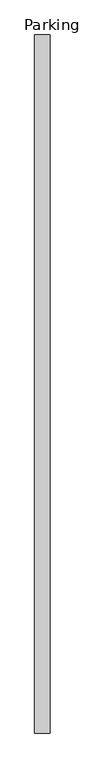
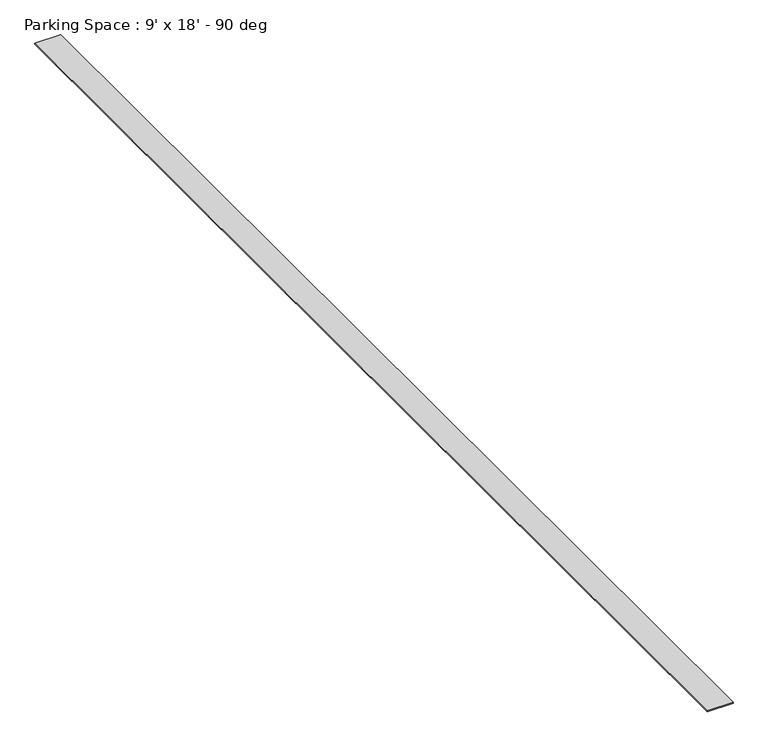
"""IFC4 building model written with IfcOpenShell, lengths in millimetres: proxy geometry, Parking Space : 9' x 18' - 90 deg."""

from ifc_helpers import new_model, si_unit, origin, origin_with_axes, place, context, project, spatial, polyline, outline, extrude, source, transform, mapped, element, save


def parking_space_9_x_18_90_deg_85bc4432(model_context):
    return source(origin(), model_context, "Body", "SweptSolid", [
        extrude(outline(polyline([(-50.8, 0.0), (50.8, 0.0), (50.8, -4572.0), (-50.8, -4572.0), (-50.8, 0.0)])), origin_with_axes(), (0.0, 0.0, 1.0), 3.175),
    ])


if __name__ == "__main__":
    model = new_model("IFC4")
    model_context = context("Model", 3, world=origin())
    ifc_project = project(units=[si_unit("LENGTHUNIT", "METRE", prefix="MILLI")], contexts=[model_context])
    site = spatial("IfcSite", under=ifc_project)
    building = spatial("IfcBuilding", under=site)
    placement = place(None, origin())
    parking_space_9_x_18_90_deg_shape = parking_space_9_x_18_90_deg_85bc4432(model_context)
    element("IfcBuildingElementProxy", 1, Name="Parking Space : 9' x 18' - 90 deg", ObjectType="Parking Space : 9' x 18' - 90 deg", at=placement, inside=building, context=model_context, shape_type="MappedRepresentation", body=[
        mapped(parking_space_9_x_18_90_deg_shape, transform((0.0, 0.0, 0.0), x_axis=(1.0, 0.0, 0.0), y_axis=(0.0, 1.0, 0.0), z_axis=(0.0, 0.0, 1.0))),
    ])
    save(model, "model.ifc")

# Revit data of these elements
# Type "Parking Space : 9' x 18' - 90 deg"
#   Angle = 90.00°
#   Parking Length = 14' - 0"
#   Parking Width = 9' - 0"
#   pl = 15' - 0"
#   pw = 7' - 0"
# Element 1 (IfcBuildingElementProxy, "Parking Space : 9' x 18' - 90 deg")
#   Materials on its faces: "Parking Stripe"
# Materials
#   "Parking Stripe": class "Paint", colour RGB 250 250 91, transparency 0
